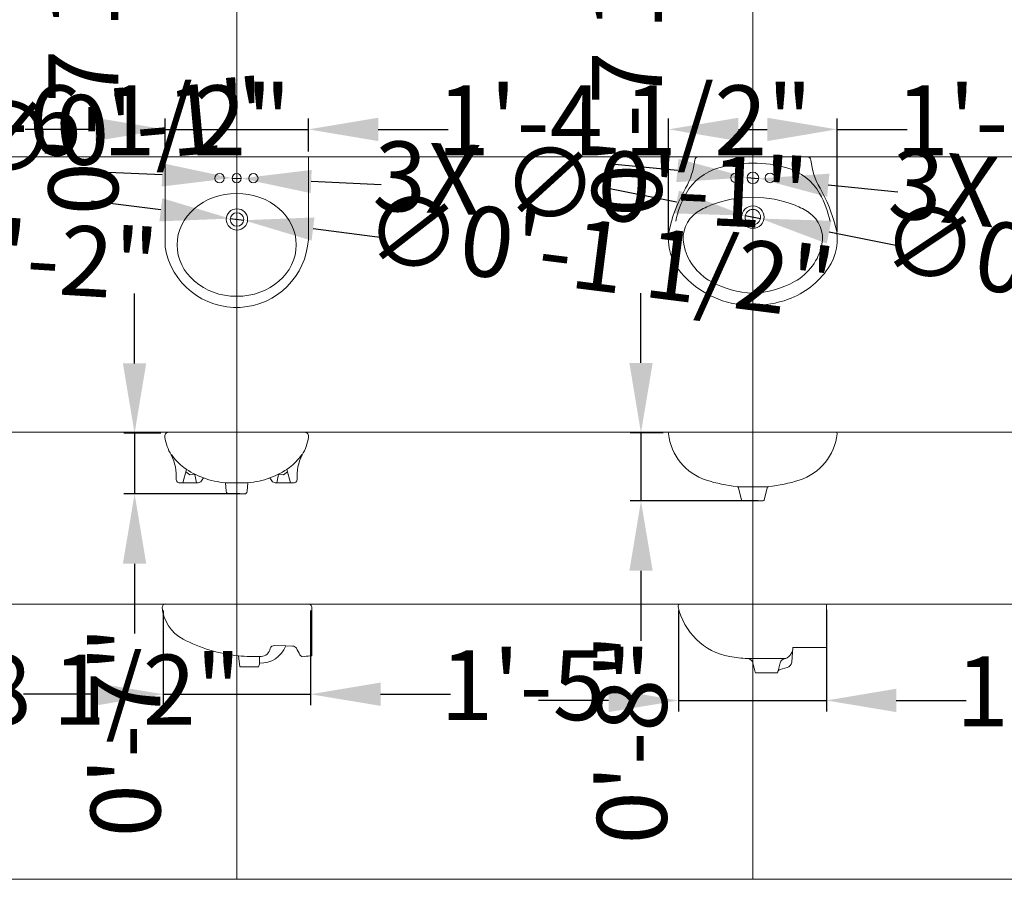
# Model space of a CAD drawing. Units: inches. Extents: x 2138 to 3265, y 2149 to 3392.
# Tile 10 of 13: x 3040 to 3153, y 3066 to 3164. Entities that reach past the tile are written whole.
import ezdxf

# ---------------------------------------------------------------- set-up
doc = ezdxf.new("R2010")
doc.units = ezdxf.units.IN
for name, color, linetype, lineweight in [('A-ANNO-DIMS', 2, 'Continuous', 18), ('A-DETL-GRID', 1, 'Continuous', 13), ('Washbasin-detail', 251, 'Continuous', 13), ('Washbasin-outline', 250, 'Continuous', 20)]:
    doc.layers.add(name, color=color, linetype=linetype, lineweight=lineweight)
doc.styles.get("Standard").update_dxf_attribs({"font": 'arial.ttf'})
doc.dimstyles.new('ISO-25', dxfattribs={"dimtxt": 8, "dimasz": 8, "dimexe": 1.25, "dimexo": 0.625, "dimtad": 0, "dimdec": 1, "dimlunit": 4, "dimtxsty": 'Standard', "dimcen": 2.5, "dimadec": 0, "dimazin": 0, "dimtfac": 1, "dimtdec": 1, "dimtmove": 0, "dimatfit": 3, "dimfxl": 1, "dimarcsym": 0})

# ---------------------------------------------------------------- blocks, each defined once
blk = doc.blocks.new('*D89')
at = {"layer": 'A-ANNO-DIMS', "color": 0, "lineweight": -2, "transparency": 16777216}
for p, q in [((3048.17, 3215.38), (3048.17, 3223.38)), ((3050.93, 3207.38), (3046.92, 3207.38)), ((3048.17, 3207.38), (3048.17, 3199.85)), ((3065.38, 3199.85), (3046.92, 3199.85)), ((3048.17, 3191.85), (3048.17, 3183.85))]:
    blk.add_line(p, q, dxfattribs=at)
at = {"layer": 'A-ANNO-DIMS', "color": 0, "transparency": 16777216}
for points in [[(3046.84, 3215.38), (3049.5, 3215.38), (3048.17, 3207.38)], [(3046.84, 3191.85), (3049.5, 3191.85), (3048.17, 3199.85)]]:
    blk.add_solid(points, dxfattribs=at)
at = {"layer": 'Defpoints', "color": 0, "transparency": 16777216}
for p in [(3051.56, 3207.38), (3048.17, 3199.85), (3066, 3199.85)]:
    blk.add_point(p, dxfattribs=at)
at = {"layer": 'A-ANNO-DIMS', "color": 0, "transparency": 16777216, "insert": (3048.17, 3163.27), "char_height": 8, "attachment_point": 5, "rotation": 90}
blk.add_mtext('0\'-7 1/2"', dxfattribs=at)
blk = doc.blocks.new('*D92')
at = {"layer": 'A-ANNO-DIMS', "color": 0, "lineweight": -2, "transparency": 16777216}
for p, q in [((3110.37, 3215.35), (3110.37, 3223.35)), ((3113.57, 3207.35), (3109.12, 3207.35)), ((3110.37, 3207.35), (3110.37, 3199.66)), ((3124.47, 3199.66), (3109.12, 3199.66)), ((3110.37, 3191.66), (3110.37, 3183.66))]:
    blk.add_line(p, q, dxfattribs=at)
at = {"layer": 'A-ANNO-DIMS', "color": 0, "transparency": 16777216}
for points in [[(3109.04, 3215.35), (3111.7, 3215.35), (3110.37, 3207.35)], [(3109.04, 3191.66), (3111.7, 3191.66), (3110.37, 3199.66)]]:
    blk.add_solid(points, dxfattribs=at)
at = {"layer": 'Defpoints', "color": 0, "transparency": 16777216}
for p in [(3114.19, 3207.35), (3110.37, 3199.66), (3125.1, 3199.66)]:
    blk.add_point(p, dxfattribs=at)
at = {"layer": 'A-ANNO-DIMS', "color": 0, "transparency": 16777216, "insert": (3110.37, 3163.08), "char_height": 8, "attachment_point": 5, "rotation": 90}
blk.add_mtext('0\'-7 1/2"', dxfattribs=at)
blk = doc.blocks.new('*D99')
at = {"layer": 'A-ANNO-DIMS', "color": 0, "lineweight": -2, "transparency": 16777216}
for p, q in [((2990.46, 3138.73), (2990.46, 3152.87)), ((3020.79, 3138.73), (3020.79, 3152.87)), ((2998.46, 3151.62), (3012.79, 3151.62)), ((3020.79, 3151.62), (3028.79, 3151.62))]:
    blk.add_line(p, q, dxfattribs=at)
at = {"layer": 'A-ANNO-DIMS', "color": 0, "transparency": 16777216}
for points in [[(2998.46, 3152.95), (2998.46, 3150.28), (2990.46, 3151.62)], [(3012.79, 3152.95), (3012.79, 3150.28), (3020.79, 3151.62)]]:
    blk.add_solid(points, dxfattribs=at)
at = {"layer": 'Defpoints', "color": 0, "transparency": 16777216}
for p in [(3020.79, 3151.62), (2990.46, 3138.1), (3020.79, 3138.1)]:
    blk.add_point(p, dxfattribs=at)
at = {"layer": 'A-ANNO-DIMS', "color": 0, "transparency": 16777216, "insert": (3049.44, 3151.62), "char_height": 8, "attachment_point": 5}
blk.add_mtext('2\'-6 1/2"', dxfattribs=at)
blk = doc.blocks.new('*D101')
at = {"layer": 'A-ANNO-DIMS', "color": 0, "lineweight": -2, "transparency": 16777216}
for p, q in [((2995.19, 3096.14), (2995.19, 3085.21)), ((3015.5, 3096.19), (3015.5, 3085.21)), ((3003.19, 3086.46), (3007.5, 3086.46)), ((3015.5, 3086.46), (3023.5, 3086.46))]:
    blk.add_line(p, q, dxfattribs=at)
at = {"layer": 'A-ANNO-DIMS', "color": 0, "transparency": 16777216}
for points in [[(3003.19, 3087.79), (3003.19, 3085.13), (2995.19, 3086.46)], [(3007.5, 3087.79), (3007.5, 3085.13), (3015.5, 3086.46)]]:
    blk.add_solid(points, dxfattribs=at)
at = {"layer": 'Defpoints', "color": 0, "transparency": 16777216}
for p in [(2995.19, 3096.77), (3015.5, 3096.81), (3015.5, 3086.46)]:
    blk.add_point(p, dxfattribs=at)
at = {"layer": 'A-ANNO-DIMS', "color": 0, "transparency": 16777216, "insert": (3043.7, 3086.46), "char_height": 8, "attachment_point": 5}
blk.add_mtext('1\'-8 1/2"', dxfattribs=at)
blk = doc.blocks.new('*D102')
at = {"layer": 'A-ANNO-DIMS', "color": 0, "lineweight": -2, "transparency": 16777216}
for p, q in [((3056.49, 3149.09), (3056.49, 3152.87)), ((3072.88, 3149.09), (3072.88, 3152.87)), ((3048.49, 3151.62), (3040.49, 3151.62)), ((3056.49, 3151.62), (3072.88, 3151.62)), ((3080.88, 3151.62), (3088.88, 3151.62))]:
    blk.add_line(p, q, dxfattribs=at)
at = {"layer": 'A-ANNO-DIMS', "color": 0, "transparency": 16777216}
for points in [[(3048.49, 3152.95), (3048.49, 3150.28), (3056.49, 3151.62)], [(3080.88, 3152.95), (3080.88, 3150.28), (3072.88, 3151.62)]]:
    blk.add_solid(points, dxfattribs=at)
at = {"layer": 'Defpoints', "color": 0, "transparency": 16777216}
for p in [(3072.88, 3151.62), (3056.49, 3148.47), (3072.88, 3148.47)]:
    blk.add_point(p, dxfattribs=at)
at = {"layer": 'A-ANNO-DIMS', "color": 0, "transparency": 16777216, "insert": (3109.08, 3151.62), "char_height": 8, "attachment_point": 5}
blk.add_mtext('1\'-4 1/2"', dxfattribs=at)
blk = doc.blocks.new('*D103')
at = {"layer": 'A-ANNO-DIMS', "color": 0, "lineweight": -2, "transparency": 16777216}
for p, q in [((3053, 3124.84), (3053, 3132.84)), ((3055.99, 3116.84), (3051.75, 3116.84)), ((3053, 3116.84), (3053, 3109.91)), ((3065.05, 3109.91), (3051.75, 3109.91)), ((3053, 3101.91), (3053, 3093.91))]:
    blk.add_line(p, q, dxfattribs=at)
at = {"layer": 'A-ANNO-DIMS', "color": 0, "transparency": 16777216}
for points in [[(3051.66, 3124.84), (3054.33, 3124.84), (3053, 3116.84)], [(3051.66, 3101.91), (3054.33, 3101.91), (3053, 3109.91)]]:
    blk.add_solid(points, dxfattribs=at)
at = {"layer": 'Defpoints', "color": 0, "transparency": 16777216}
for p in [(3056.61, 3116.84), (3053, 3109.91), (3065.67, 3109.91)]:
    blk.add_point(p, dxfattribs=at)
at = {"layer": 'A-ANNO-DIMS', "color": 0, "transparency": 16777216, "insert": (3053, 3082.66), "char_height": 8, "attachment_point": 5, "rotation": 90}
blk.add_mtext('0\'-7"', dxfattribs=at)
blk = doc.blocks.new('*D104')
at = {"layer": 'A-ANNO-DIMS', "color": 0, "lineweight": -2, "transparency": 16777216}
for p, q in [((3056.27, 3096.57), (3056.27, 3085.72)), ((3073.14, 3096.56), (3073.14, 3085.72)), ((3048.27, 3086.97), (3040.27, 3086.97)), ((3056.27, 3086.97), (3073.14, 3086.97)), ((3081.14, 3086.97), (3089.14, 3086.97))]:
    blk.add_line(p, q, dxfattribs=at)
at = {"layer": 'A-ANNO-DIMS', "color": 0, "transparency": 16777216}
for points in [[(3048.27, 3088.31), (3048.27, 3085.64), (3056.27, 3086.97)], [(3081.14, 3088.31), (3081.14, 3085.64), (3073.14, 3086.97)]]:
    blk.add_solid(points, dxfattribs=at)
at = {"layer": 'Defpoints', "color": 0, "transparency": 16777216}
for p in [(3056.27, 3097.19), (3073.14, 3097.19), (3073.14, 3086.97)]:
    blk.add_point(p, dxfattribs=at)
at = {"layer": 'A-ANNO-DIMS', "color": 0, "transparency": 16777216, "insert": (3100.02, 3086.97), "char_height": 8, "attachment_point": 5}
blk.add_mtext('1\'-5"', dxfattribs=at)
blk = doc.blocks.new('*D105')
at = {"layer": 'A-ANNO-DIMS', "color": 0, "lineweight": -2, "transparency": 16777216}
for p, q in [((3114.09, 3139.73), (3114.09, 3152.87)), ((3133.38, 3139.88), (3133.38, 3152.87)), ((3122.09, 3151.62), (3125.38, 3151.62)), ((3133.38, 3151.62), (3141.38, 3151.62))]:
    blk.add_line(p, q, dxfattribs=at)
at = {"layer": 'A-ANNO-DIMS', "color": 0, "transparency": 16777216}
for points in [[(3122.09, 3152.95), (3122.09, 3150.28), (3114.09, 3151.62)], [(3125.38, 3152.95), (3125.38, 3150.28), (3133.38, 3151.62)]]:
    blk.add_solid(points, dxfattribs=at)
at = {"layer": 'Defpoints', "color": 0, "transparency": 16777216}
for p in [(3133.38, 3151.62), (3114.09, 3139.11), (3133.38, 3139.26)]:
    blk.add_point(p, dxfattribs=at)
at = {"layer": 'A-ANNO-DIMS', "color": 0, "transparency": 16777216, "insert": (3161.58, 3151.62), "char_height": 8, "attachment_point": 5}
blk.add_mtext('1\'-7 1/2"', dxfattribs=at)
blk = doc.blocks.new('*D106')
at = {"layer": 'A-ANNO-DIMS', "color": 0, "lineweight": -2, "transparency": 16777216}
for p, q in [((3110.94, 3124.89), (3110.94, 3132.89)), ((3113.49, 3116.89), (3109.69, 3116.89)), ((3110.94, 3116.89), (3110.94, 3109.1)), ((3124.34, 3109.1), (3109.69, 3109.1)), ((3110.94, 3101.1), (3110.94, 3093.1))]:
    blk.add_line(p, q, dxfattribs=at)
at = {"layer": 'A-ANNO-DIMS', "color": 0, "transparency": 16777216}
for points in [[(3109.61, 3124.89), (3112.28, 3124.89), (3110.94, 3116.89)], [(3109.61, 3101.1), (3112.28, 3101.1), (3110.94, 3109.1)]]:
    blk.add_solid(points, dxfattribs=at)
at = {"layer": 'Defpoints', "color": 0, "transparency": 16777216}
for p in [(3114.11, 3116.89), (3110.94, 3109.1), (3124.96, 3109.1)]:
    blk.add_point(p, dxfattribs=at)
at = {"layer": 'A-ANNO-DIMS', "color": 0, "transparency": 16777216, "insert": (3110.94, 3081.85), "char_height": 8, "attachment_point": 5, "rotation": 90}
blk.add_mtext('0\'-8"', dxfattribs=at)
blk = doc.blocks.new('*D107')
at = {"layer": 'A-ANNO-DIMS', "color": 0, "lineweight": -2, "transparency": 16777216}
for p, q in [((3115.23, 3096.57), (3115.23, 3085.01)), ((3132.15, 3096.63), (3132.15, 3085.01)), ((3107.23, 3086.26), (3099.23, 3086.26)), ((3115.23, 3086.26), (3132.15, 3086.26)), ((3140.15, 3086.26), (3148.15, 3086.26))]:
    blk.add_line(p, q, dxfattribs=at)
at = {"layer": 'A-ANNO-DIMS', "color": 0, "transparency": 16777216}
for points in [[(3107.23, 3087.6), (3107.23, 3084.93), (3115.23, 3086.26)], [(3140.15, 3087.6), (3140.15, 3084.93), (3132.15, 3086.26)]]:
    blk.add_solid(points, dxfattribs=at)
at = {"layer": 'Defpoints', "color": 0, "transparency": 16777216}
for p in [(3115.23, 3097.2), (3132.15, 3097.25), (3132.15, 3086.26)]:
    blk.add_point(p, dxfattribs=at)
at = {"layer": 'A-ANNO-DIMS', "color": 0, "transparency": 16777216, "insert": (3159.03, 3086.26), "char_height": 8, "attachment_point": 5}
blk.add_mtext('1\'-5"', dxfattribs=at)
blk = doc.blocks.new('*D132')
at = {"layer": 'A-ANNO-DIMS', "color": 0, "lineweight": -2, "transparency": 16777216}
for p, q in [((3019.38, 3147.98), (3011.42, 3147.24)), ((2994.46, 3145.69), (2986.49, 3144.95)), ((3002.43, 3146.42), (3003.45, 3146.51))]:
    blk.add_line(p, q, dxfattribs=at)
at = {"layer": 'A-ANNO-DIMS', "color": 0, "transparency": 16777216}
for points in [[(3011.29, 3148.57), (3011.54, 3145.92), (3003.45, 3146.51)], [(2994.34, 3147.01), (2994.58, 3144.36), (3002.43, 3146.42)]]:
    blk.add_solid(points, dxfattribs=at)
at = {"layer": 'Defpoints', "color": 0, "transparency": 16777216}
for p in [(3002.43, 3146.42), (3003.45, 3146.51)]:
    blk.add_point(p, dxfattribs=at)
at = {"layer": 'A-ANNO-DIMS', "color": 0, "transparency": 16777216, "insert": (3043.34, 3150.18), "char_height": 8, "attachment_point": 5, "rotation": 5.2513}
blk.add_mtext('2X ∅0\'-1"', dxfattribs=at)
blk = doc.blocks.new('*D133')
at = {"layer": 'A-ANNO-DIMS', "color": 0, "lineweight": -2, "transparency": 16777216}
for p, q in [((2996.7, 3138.67), (2988.72, 3139.17)), ((3004.68, 3138.17), (3006.57, 3138.05)), ((3022.54, 3137.05), (3014.56, 3137.55))]:
    blk.add_line(p, q, dxfattribs=at)
at = {"layer": 'A-ANNO-DIMS', "color": 0, "transparency": 16777216}
for points in [[(2996.78, 3140), (2996.62, 3137.34), (3004.68, 3138.17)], [(3014.64, 3138.88), (3014.47, 3136.22), (3006.57, 3138.05)]]:
    blk.add_solid(points, dxfattribs=at)
at = {"layer": 'Defpoints', "color": 0, "transparency": 16777216}
for p in [(3004.68, 3138.17), (3006.57, 3138.05)]:
    blk.add_point(p, dxfattribs=at)
at = {"layer": 'A-ANNO-DIMS', "color": 0, "transparency": 16777216, "insert": (3038.12, 3136.08), "char_height": 8, "attachment_point": 5, "rotation": 356.4158}
blk.add_mtext('∅0\'-2"', dxfattribs=at)
blk = doc.blocks.new('*D134')
at = {"layer": 'A-ANNO-DIMS', "color": 0, "lineweight": -2, "transparency": 16777216}
for p, q in [((3056.16, 3146.41), (3048.17, 3146.77)), ((3064.15, 3146.05), (3065.21, 3146.01)), ((3081.2, 3145.29), (3073.2, 3145.65))]:
    blk.add_line(p, q, dxfattribs=at)
at = {"layer": 'A-ANNO-DIMS', "color": 0, "transparency": 16777216}
for points in [[(3056.22, 3147.74), (3056.1, 3145.08), (3064.15, 3146.05)], [(3073.26, 3146.98), (3073.15, 3144.32), (3065.21, 3146.01)]]:
    blk.add_solid(points, dxfattribs=at)
at = {"layer": 'Defpoints', "color": 0, "transparency": 16777216}
for p in [(3064.15, 3146.05), (3065.21, 3146.01)]:
    blk.add_point(p, dxfattribs=at)
at = {"layer": 'A-ANNO-DIMS', "color": 0, "transparency": 16777216, "insert": (3105.16, 3144.22), "char_height": 8, "attachment_point": 5, "rotation": 357.4417}
blk.add_mtext('3X ∅0\'-1"', dxfattribs=at)
blk = doc.blocks.new('*D135')
at = {"layer": 'A-ANNO-DIMS', "color": 0, "lineweight": -2, "transparency": 16777216}
for p, q in [((3056, 3142.41), (3048.07, 3143.41)), ((3063.94, 3141.41), (3065.48, 3141.22)), ((3081.35, 3139.22), (3073.42, 3140.22))]:
    blk.add_line(p, q, dxfattribs=at)
at = {"layer": 'A-ANNO-DIMS', "color": 0, "transparency": 16777216}
for points in [[(3056.17, 3143.73), (3055.84, 3141.09), (3063.94, 3141.41)], [(3073.58, 3141.54), (3073.25, 3138.89), (3065.48, 3141.22)]]:
    blk.add_solid(points, dxfattribs=at)
at = {"layer": 'Defpoints', "color": 0, "transparency": 16777216}
for p in [(3063.94, 3141.41), (3065.48, 3141.22)]:
    blk.add_point(p, dxfattribs=at)
at = {"layer": 'A-ANNO-DIMS', "color": 0, "transparency": 16777216, "insert": (3106.09, 3136.1), "char_height": 8, "attachment_point": 5, "rotation": 352.8242}
blk.add_mtext('∅0\'-1 1/2"', dxfattribs=at)
blk = doc.blocks.new('*D136')
at = {"layer": 'A-ANNO-DIMS', "color": 0, "lineweight": -2, "transparency": 16777216}
for p, q in [((3115.11, 3146.91), (3107.15, 3147.69)), ((3123.07, 3146.13), (3124.4, 3146)), ((3140.33, 3144.45), (3132.37, 3145.22))]:
    blk.add_line(p, q, dxfattribs=at)
at = {"layer": 'A-ANNO-DIMS', "color": 0, "transparency": 16777216}
for points in [[(3115.24, 3148.24), (3114.98, 3145.58), (3123.07, 3146.13)], [(3132.5, 3146.55), (3132.24, 3143.9), (3124.4, 3146)]]:
    blk.add_solid(points, dxfattribs=at)
at = {"layer": 'Defpoints', "color": 0, "transparency": 16777216}
for p in [(3123.07, 3146.13), (3124.4, 3146)]:
    blk.add_point(p, dxfattribs=at)
at = {"layer": 'A-ANNO-DIMS', "color": 0, "transparency": 16777216, "insert": (3173.48, 3141.21), "char_height": 8, "attachment_point": 5, "rotation": 354.4214}
blk.add_mtext('3X ∅0\'-1 1/2"', dxfattribs=at)
blk = doc.blocks.new('*D137')
at = {"layer": 'A-ANNO-DIMS', "color": 0, "lineweight": -2, "transparency": 16777216}
for p, q in [((3115.02, 3143.3), (3107.17, 3144.86)), ((3122.87, 3141.75), (3124.61, 3141.41)), ((3140.3, 3138.3), (3132.46, 3139.85))]:
    blk.add_line(p, q, dxfattribs=at)
at = {"layer": 'A-ANNO-DIMS', "color": 0, "transparency": 16777216}
for points in [[(3115.28, 3144.61), (3114.76, 3142), (3122.87, 3141.75)], [(3132.71, 3141.16), (3132.2, 3138.55), (3124.61, 3141.41)]]:
    blk.add_solid(points, dxfattribs=at)
at = {"layer": 'Defpoints', "color": 0, "transparency": 16777216}
for p in [(3122.87, 3141.75), (3124.61, 3141.41)]:
    blk.add_point(p, dxfattribs=at)
at = {"layer": 'A-ANNO-DIMS', "color": 0, "transparency": 16777216, "insert": (3155.62, 3135.27), "char_height": 8, "attachment_point": 5, "rotation": 348.8088}
blk.add_mtext('∅0\'-2"', dxfattribs=at)

msp = doc.modelspace()

# ---------------------------------------------------------------- linework, layer by layer
at = {"layer": 'A-DETL-GRID'}
for p, q in [((3064.68, 3148.47), (3064.68, 3239.02)), ((3123.74, 3148.47), (3123.74, 3239.02)), ((2828.46, 3148.47), (3241.85, 3148.47)), ((2828.46, 3148.47), (3241.85, 3148.47)), ((3064.68, 3065.79), (3064.68, 3148.47)), ((3123.74, 3065.79), (3123.74, 3148.47)), ((2828.46, 3116.97), (3241.85, 3116.97)), ((2828.46, 3097.29), (3241.85, 3097.29)), ((2828.46, 3065.79), (3241.85, 3065.79))]:
    msp.add_line(p, q, dxfattribs=at)
at = {"layer": 'Washbasin-detail'}
for p, q in [((3121.99, 3110.71), (3123.74, 3110.71)), ((3125.49, 3110.71), (3123.74, 3110.71)), ((3123.11, 3091.07), (3127.5, 3091.07)), ((3126.61, 3089.5), (3126.86, 3090.55))]:
    msp.add_line(p, q, dxfattribs=at)
for points in [[(3060.88, 3111.73), (3060.59, 3111.27), (3060.26, 3111.18), (3058.22, 3111.16, -0.357028), (3057.75, 3111.53, 0.138574), (3057.19, 3114.37, 270.662595)], [(3068.48, 3111.73), (3068.77, 3111.27), (3069.1, 3111.18), (3071.14, 3111.16, 0.357028), (3071.61, 3111.53, -0.138574), (3072.17, 3114.37, -270.662595)], [(3063.41, 3111.18), (3063.48, 3110.2, 0.393459), (3063.81, 3109.89), (3064.68, 3109.89)], [(3065.95, 3111.18), (3065.88, 3110.2, -0.393459), (3065.55, 3109.89), (3064.68, 3109.89)], [(3067.29, 3090.53, 0.315838), (3070.3, 3092.5, -1.057911)]]:
    msp.add_lwpolyline(points, format="xyb", dxfattribs=at)
for points in [[(3058.51, 3111.16), (3058.95, 3112.71)], [(3058.87, 3112.42), (3059.32, 3112.07), (3059.93, 3112.14)], [(3059.89, 3112.13), (3060.1, 3111.18)], [(3069.47, 3112.13), (3069.26, 3111.18)], [(3070.49, 3112.42), (3070.03, 3112.07), (3069.43, 3112.14)], [(3070.85, 3111.16), (3070.41, 3112.71)], [(3064.9, 3091.37), (3065.05, 3090.12), (3067.16, 3090.12), (3067.29, 3090.4)], [(3067.29, 3090.4), (3067.31, 3091.3)]]:
    msp.add_lwpolyline(points, dxfattribs=at)
for centre, radius in [((3121.77, 3146.07), 0.551), ((3125.71, 3146.07), 0.551), ((3062.72, 3146.03), 0.53), ((3064.68, 3146.03), 0.53), ((3066.59, 3146.03), 0.53), ((3064.71, 3141.31), 1.22), ((3064.71, 3141.31), 0.775)]:
    msp.add_circle(centre, radius, dxfattribs=at)
for centre, radius, start, end in [((3123.74, 3133.59), 14.17, 90, 105.998), ((3123.74, 3133.59), 14.17, 74.002, 90), ((3121.57, 3141.16), 6.3, 105.998, 150.1904), ((3123.74, 3146.07), 0.669, 90, 270), ((3123.74, 3146.07), 0.669, 270, 90), ((3125.91, 3141.16), 6.3, 29.8096, 74.002), ((3125.33, 3139), 10.63, 150.1904, 168.5867), ((3122.15, 3139), 10.63, 11.4133, 29.8096), ((3123.74, 3141.58), 1.28, 90, 270), ((3123.74, 3141.58), 0.886, 90, 270), ((3123.74, 3141.58), 1.28, 270, 90), ((3123.74, 3141.58), 0.886, 270, 90), ((3126.98, 3092.3), 1.34, 292.7471, 1.3462), ((3127.51, 3090.4), 0.669, 91.18, 166.6297)]:
    msp.add_arc(centre, radius, start, end, dxfattribs=at)
at = {"layer": 'Washbasin-outline'}
for p, q in [((3117.48, 3148.47), (3118.88, 3148.47)), ((3118.88, 3148.47), (3123.74, 3148.47)), ((3129.99, 3148.47), (3123.74, 3148.47)), ((3129.99, 3148.47), (3123.74, 3148.47)), ((3114.25, 3116.97), (3123.74, 3116.97)), ((3133.23, 3116.97), (3123.74, 3116.97)), ((3122.44, 3109.19), (3122.11, 3110.58)), ((3125.04, 3109.19), (3125.37, 3110.58)), ((3122.55, 3109.1), (3123.74, 3109.1)), ((3124.92, 3109.1), (3123.74, 3109.1)), ((3072.82, 3097.27), (3056.55, 3097.3)), ((3132.06, 3097.29), (3115.41, 3097.29)), ((3132.18, 3092.45), (3132.18, 3097.17)), ((3073.28, 3091.37), (3073.28, 3096.89)), ((3128.32, 3092.33), (3128.19, 3090.65)), ((3132.06, 3092.33), (3128.32, 3092.33)), ((3123.99, 3089.5), (3123.74, 3090.55)), ((3126.5, 3089.41), (3124.11, 3089.41)), ((3126.87, 3089.81), (3127.66, 3090.02))]:
    msp.add_line(p, q, dxfattribs=at)
for points in [[(3056.49, 3148.47), (3072.88, 3148.47)], [(3070.3, 3092.5), (3071.08, 3092.48)]]:
    msp.add_lwpolyline(points, dxfattribs=at)
for points in [[(3056.49, 3148.47), (3056.49, 3138.13, 0.894265), (3072.88, 3139.03), (3072.88, 3148.47)], [(3064.67, 3116.97), (3056.88, 3116.97, 0.426353), (3056.46, 3116.39, 0.097827), (3057.19, 3114.37, 0.137679)], [(3064.68, 3116.97), (3072.47, 3116.97, -0.426353), (3072.9, 3116.39, -0.097827), (3072.17, 3114.37, -0.067753)], [(3057.24, 3114.4, 0.094323), (3058.64, 3112.92, 0.068248), (3060.88, 3111.73, 0.459681)], [(3072.12, 3114.4, -0.094323), (3070.71, 3112.92, -0.068248), (3068.48, 3111.73, -0.459681)], [(3060.88, 3111.73, 0.069778), (3063.41, 3111.18, 0.459681)], [(3068.48, 3111.73, -0.069778), (3065.95, 3111.18, -0.459681)], [(3063.41, 3111.18, 0.034215), (3064.68, 3111.17, 0.459681)], [(3065.95, 3111.18, -0.034215), (3064.68, 3111.17, -0.459681)], [(3058.54, 3093.29, 0.096563), (3064.9, 3091.37, 0.340427)], [(3064.9, 3091.37, 0.037087), (3067.47, 3091.3, 0.340427), (3068.53, 3092.2, -0.381938), (3069, 3092.54), (3070.3, 3092.5)]]:
    msp.add_lwpolyline(points, format="xyb", dxfattribs=at)
for centre, radius, start, end in [((3108.87, 3149.01), 8.27, 330.1677, 353.768), ((3117.48, 3148.07), 0.394, 90, 173.768), ((3129.99, 3148.07), 0.394, 4.096, 90), ((3138.6, 3149.01), 8.27, 186.232, 209.8323), ((3131.07, 3136.28), 17.32, 150.1677, 165.9365), ((3116.4, 3136.28), 17.32, 14.0635, 29.8323), ((3123.74, 3130.46), 13.39, 90, 111.253), ((3123.74, 3130.46), 13.39, 68.747, 90), ((3119.3, 3139.17), 3.54, 124.2728, 191.4009), ((3121.74, 3135.59), 7.87, 111.253, 124.2728), ((3125.74, 3135.59), 7.87, 55.7272, 68.747), ((3128.17, 3139.17), 3.54, 348.5991, 55.7272), ((3120, 3139.06), 5.91, 165.9365, 220.016), ((3127.48, 3139.06), 5.91, 325.7528, 14.0635), ((3122, 3139.72), 6.3, 191.4009, 241.0819), ((3125.47, 3139.72), 6.3, 298.9181, 348.5991), ((3124.55, 3141.05), 9.45, 290.0846, 325.7528), ((3123.62, 3142.1), 10.63, 220.016, 270.6571), ((3124.1, 3143.51), 10.63, 241.0819, 268.0649), ((3123.38, 3143.51), 10.63, 271.9351, 298.9181), ((3123.74, 3143.27), 11.81, 270, 290.0846), ((3114.25, 3116.81), 0.157, 90, 186.0692), ((3120.36, 3117.46), 6.3, 186.0692, 252.1399), ((3127.12, 3117.46), 6.3, 287.8601, 353.9308), ((3133.23, 3116.81), 0.157, 353.9308, 90), ((3123.74, 3127.96), 17.32, 252.1399, 264.0265), ((3121.92, 3110.53), 0.197, 13.3925, 84.0265), ((3125.56, 3110.53), 0.197, 95.9735, 166.6075), ((3123.74, 3127.96), 17.32, 275.9735, 287.8601), ((3122.55, 3109.22), 0.118, 193.3925, 270), ((3124.92, 3109.22), 0.118, 270, 346.6075), ((3056.55, 3096.9), 0.404, 90, 177.402), ((3072.89, 3096.89), 0.392, 0, 100.7346), ((3115.41, 3097.05), 0.236, 90, 192.5798), ((3122.48, 3098.63), 7.48, 192.5798, 259.3296), ((3132.06, 3097.17), 0.118, 0, 90), ((3060.61, 3097.25), 4.47, 184.3051, 242.4354), ((3071.07, 3091.96), 0.519, 31.4575, 89.0913), ((3064.6, 3088.01), 8.1, 25.4658, 31.4575), ((3072.29, 3091.67), 0.414, 205.4658, 287.3083), ((3073.44, 3085.78), 5.59, 91.6272, 100.5944), ((3132.06, 3092.45), 0.118, 270, 0), ((3123.36, 3103.27), 12.2, 259.3296, 268.82), ((3123.09, 3090.4), 0.669, 13.3703, 88.82), ((3127.48, 3090.7), 0.709, 284.89, 355.4375), ((3124.11, 3089.53), 0.118, 193.3925, 270), ((3126.5, 3089.49), 0.0787, 270, 351.911), ((3126.97, 3089.43), 0.394, 104.89, 171.911)]:
    msp.add_arc(centre, radius, start, end, dxfattribs=at)
msp.add_ellipse((3064.68, 3138.4), major_axis=(-6.82, 0), ratio=0.863139, dxfattribs=at)

# ---------------------------------------------------------------- dimensions: what is measured, and where the dimension line sits
at = {"layer": 'A-ANNO-DIMS'}
for base, p1, p2, picture, middle in [((3048.17, 3199.85), (3051.56, 3207.38), (3066, 3199.85), '*D89', (3048.17, 3163.27)), ((3110.37, 3199.66), (3114.19, 3207.35), (3125.1, 3199.66), '*D92', (3110.37, 3163.08)), ((3053, 3109.91), (3056.61, 3116.84), (3065.67, 3109.91), '*D103', (3053, 3082.66)), ((3110.94, 3109.1), (3114.11, 3116.89), (3124.96, 3109.1), '*D106', (3110.94, 3081.85))]:
    dim = msp.add_linear_dim(base=base, p1=p1, p2=p2, angle=90, dimstyle='ISO-25', override={"dimdec": 1, "dimlfac": 1, "dimrnd": 0, "dimzin": 1, "dimdsep": 46, "dimlunit": 4, "dimfrac": 2}, dxfattribs=at)
    dim.commit()
    dim.dimension.update_dxf_attribs({"geometry": picture, "text_midpoint": middle})
dim = msp.add_diameter_dim_2p(p1=(3002.43, 3146.42), p2=(3003.45, 3146.51), text='2X <>', dimstyle='ISO-25', override={"dimdec": 1, "dimlfac": 1, "dimrnd": 0, "dimzin": 1, "dimdsep": 46, "dimlunit": 4, "dimfrac": 2}, dxfattribs=at)
dim.commit()
dim.dimension.update_dxf_attribs({"geometry": '*D132', "text_midpoint": (3043.34, 3150.18)})
for base, p1, p2, picture, middle in [((3020.79, 3151.62), (2990.46, 3138.1), (3020.79, 3138.1), '*D99', (3049.44, 3151.62)), ((3072.88, 3151.62), (3056.49, 3148.47), (3072.88, 3148.47), '*D102', (3109.08, 3151.62)), ((3133.38, 3151.62), (3114.09, 3139.11), (3133.38, 3139.26), '*D105', (3161.58, 3151.62)), ((3015.5, 3086.46), (2995.19, 3096.77), (3015.5, 3096.81), '*D101', (3043.7, 3086.46)), ((3073.14, 3086.97), (3056.27, 3097.19), (3073.14, 3097.19), '*D104', (3100.02, 3086.97)), ((3132.15, 3086.26), (3115.23, 3097.2), (3132.15, 3097.25), '*D107', (3159.03, 3086.26))]:
    dim = msp.add_linear_dim(base=base, p1=p1, p2=p2, dimstyle='ISO-25', override={"dimdec": 1, "dimlfac": 1, "dimrnd": 0, "dimzin": 1, "dimdsep": 46, "dimlunit": 4, "dimfrac": 2}, dxfattribs=at)
    dim.commit()
    dim.dimension.update_dxf_attribs({"geometry": picture, "text_midpoint": middle})
for p1, p2, picture, middle in [((3123.07, 3146.13), (3124.4, 3146), '*D136', (3173.48, 3141.21)), ((3064.15, 3146.05), (3065.21, 3146.01), '*D134', (3105.16, 3144.22))]:
    dim = msp.add_diameter_dim_2p(p1=p1, p2=p2, text='3X <>', dimstyle='ISO-25', override={"dimdec": 1, "dimlfac": 1, "dimrnd": 0, "dimzin": 1, "dimdsep": 46, "dimlunit": 4, "dimfrac": 2}, dxfattribs=at)
    dim.commit()
    dim.dimension.update_dxf_attribs({"geometry": picture, "text_midpoint": middle, "dimtype": 163})
for p1, p2, picture, middle in [((3063.94, 3141.41), (3065.48, 3141.22), '*D135', (3106.09, 3136.1)), ((3122.87, 3141.75), (3124.61, 3141.41), '*D137', (3155.62, 3135.27)), ((3004.68, 3138.17), (3006.57, 3138.05), '*D133', (3038.12, 3136.08))]:
    dim = msp.add_diameter_dim_2p(p1=p1, p2=p2, dimstyle='ISO-25', override={"dimdec": 1, "dimlfac": 1, "dimrnd": 0, "dimzin": 1, "dimdsep": 46, "dimlunit": 4, "dimfrac": 2}, dxfattribs=at)
    dim.commit()
    dim.dimension.update_dxf_attribs({"geometry": picture, "text_midpoint": middle})

doc.saveas('drawing.dxf')
